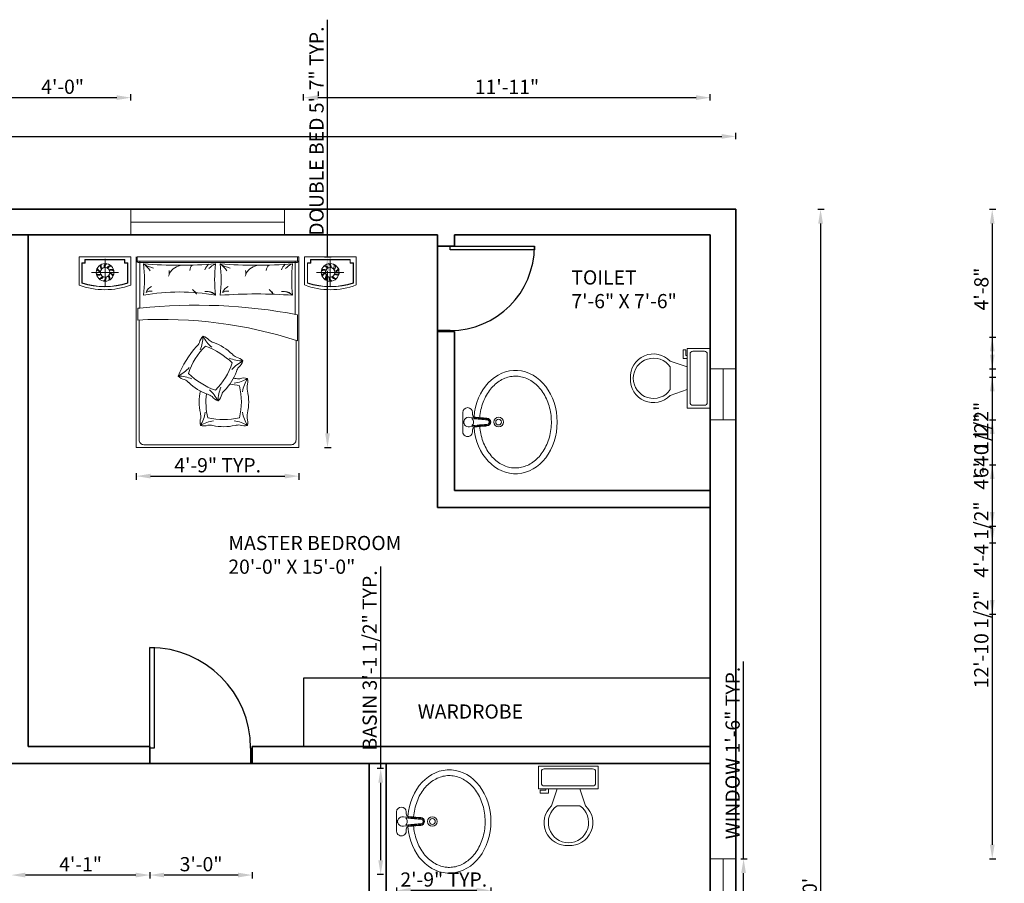
# Model space of a CAD drawing. Units: inches. Extents: x -48 to 817, y -530 to 78.
# Tile 7 of 7: x 470 to 817, y -225 to 78. Entities that reach past the tile are written whole.
import ezdxf

# ---------------------------------------------------------------- set-up
doc = ezdxf.new("R2010")
doc.units = ezdxf.units.IN
for name, color, linetype, lineweight in [('A-ANNO-DIMS', 2, 'Continuous', 18), ('A-AREA-IDEN', 7, 'Continuous', 18), ('A-DOOR', 3, 'Continuous', 25), ('A-FLOR-CASE', 8, 'Continuous', 25), ('A-FLOR-FIXT', 9, 'Continuous', 18), ('A-GLAZ', 4, 'Continuous', 18), ('A-WALL', 7, 'Continuous', 35), ('furn', 8, 'Continuous', 18), ('txt', 7, 'Continuous', 18)]:
    doc.layers.add(name, color=color, linetype=linetype, lineweight=lineweight)
doc.styles.get("Standard").update_dxf_attribs({"font": 'arial.ttf'})
doc.dimstyles.new('ISO-25', dxfattribs={"dimtxt": 5, "dimasz": 5, "dimexe": 1.25, "dimexo": 0.625, "dimtad": 1, "dimlunit": 3, "dimtxsty": 'Standard', "dimcen": 2.5, "dimadec": 0, "dimazin": 0, "dimtfac": 1, "dimtmove": 0, "dimatfit": 3, "dimfxl": 1, "dimfxlon": 1, "dimarcsym": 0})

# ---------------------------------------------------------------- blocks, each defined once
blk = doc.blocks.new('*U4')
for p, q in [((9.5, -6), (9.5, -2)), ((-10, -8.5), (-8, -8.5)), ((-10, -9.5), (-10, -8.5)), ((-7, -9.5), (-10, -9.5)), ((-8, -8.5), (-8, -8)), ((-7, -8), (-7, -9.5)), ((-4, -8), (-6, -14)), ((4, -8), (6, -14)), ((4, -14), (-4, -14))]:
    blk.add_line(p, q)
blk.add_lwpolyline([(10.5, -8), (10.5, 0), (-10.5, 0), (-10.5, -8)], close=True)
for points in [[(-9.5, -2), (-9.5, -6)], [(8.5, -1), (-8.5, -1)], [(-8.5, -7), (8.5, -7)]]:
    blk.add_lwpolyline(points)
for centre, radius, start, end in [((-8.625, -1.875), 0.8839, 81.8699, 188.1301), ((8.625, -1.875), 0.8839, 351.8699, 98.1301), ((-8.625, -6.125), 0.8839, 171.869898, 278.1301), ((8.625, -6.125), 0.8839, 261.8699, 8.1301), ((-0.4772, -19.9188), 8.0953, 133.01722, 273.38), ((0.0374, -19.8731), 7.127, 124.50543, 269.7), ((-0.0373, -19.8731), 7.127, 270.3, 55.4946), ((0.4773, -19.9188), 8.0953, 266.62, 46.9828)]:
    blk.add_arc(centre, radius, start, end)
blk = doc.blocks.new('*U2')
for p, q in [((0, 0), (0, -6)), ((40, 0), (40, -6))]:
    blk.add_line(p, q)
blk.add_lwpolyline([(0, 0), (0, 40), (1.75, 40), (1.75, 0)], close=True)
blk.add_arc((0, 0), 40, 0, 90)
blk = doc.blocks.new('A$C359865C9')
for p, q in [((0.26, 0.5858), (0.38, 0.5858)), ((0.26, 0.5258), (0.272, 0.5258)), ((0.368, 0.5258), (0.3809, 0.5258))]:
    blk.add_line(p, q)
for radius in [0.03, 0.018]:
    blk.add_circle((0.3201, 0.3632), radius)
for centre, radius, start, end in [((0.26, 0.5558), 0.03, 90.00613, 270.00613), ((0.32, 0.5495), 0.03, 348.15369, 191.84631), ((0.38, 0.5558), 0.03, 270.00613, 89.98161), ((0.272, 0.5078), 0.018, 0.00613, 90.00613), ((0.32, 0.5495), 0.03, 222.45226, 317.54774), ((0.368, 0.5078), 0.018, 90.00613, 180.00613), ((0.3201, 0.4358), 0.024, 180.00613, 0.00613), ((0.3201, 0.4358), 0.0204, 180.00613, 0.00613), ((0.3201, 0.4358), 0.0144, 180.00613, 0.00613)]:
    blk.add_arc(centre, radius, start, end)
at = {"extrusion": (0, 0, -1)}
blk.add_ellipse((0.3199, 0.5826), major_axis=(-0.00812, 0), ratio=0.392595, dxfattribs=at)
at = {"ltscale": 100, "extrusion": (0, 0, -1)}
blk.add_ellipse((0.3201, 0.258), major_axis=(0.3216, 0), ratio=0.80597, start_param=-1.471508, end_param=4.612925, dxfattribs=at)
for points, knots in [([(0.29, 0.5078), (0.2913, 0.4937), (0.2935, 0.4697), (0.2953, 0.4457), (0.2961, 0.4358)], [0, 0, 0, 0, 35.358253, 60.208758, 60.208758, 60.208758, 60.208758]), ([(0.2907, 0.5434), (0.2946, 0.498), (0.2952, 0.4908), (0.2965, 0.4761), (0.2971, 0.4686), (0.2983, 0.4536), (0.2989, 0.4461), (0.2995, 0.4378), (0.2996, 0.4369), (0.2996, 0.4361)], [2.511178, 2.511178, 2.511178, 2.511178, 20.495008, 20.495008, 39.297594, 39.297594, 58.10018, 58.10018, 60.208758, 60.208758, 60.208758, 60.208758]), ([(0.2979, 0.5293), (0.298, 0.528), (0.2981, 0.5267), (0.2988, 0.5184), (0.2993, 0.5127), (0.3005, 0.4986), (0.301, 0.4933), (0.3014, 0.4884), (0.3015, 0.4875), (0.3017, 0.4857), (0.3017, 0.485), (0.3019, 0.4827), (0.3021, 0.4812), (0.3026, 0.4756), (0.3029, 0.4716), (0.3037, 0.4621), (0.3041, 0.4568), (0.3049, 0.4464), (0.3053, 0.4415), (0.3056, 0.4365)], [4.643985, 4.643985, 4.643985, 4.643985, 5.282102, 5.282102, 8.976667, 8.976667, 16.365798, 16.365798, 18.536065, 18.536065, 20.434607, 20.434607, 24.231692, 24.231692, 34.371999, 34.371999, 47.807513, 47.807513, 60.208758, 60.208758, 60.208758, 60.208758]), ([(0.3422, 0.5293), (0.3421, 0.528), (0.342, 0.5267), (0.3412, 0.5184), (0.3408, 0.5127), (0.3395, 0.4986), (0.3391, 0.4933), (0.3387, 0.4884), (0.3386, 0.4875), (0.3384, 0.4857), (0.3383, 0.485), (0.3381, 0.4827), (0.338, 0.4812), (0.3375, 0.4756), (0.3372, 0.4716), (0.3364, 0.4621), (0.336, 0.4568), (0.3352, 0.4464), (0.3348, 0.4415), (0.3345, 0.4365)], [4.643985, 4.643985, 4.643985, 4.643985, 5.282102, 5.282102, 8.976667, 8.976667, 16.365798, 16.365798, 18.536065, 18.536065, 20.434607, 20.434607, 24.231692, 24.231692, 34.371999, 34.371999, 47.807513, 47.807513, 60.208758, 60.208758, 60.208758, 60.208758]), ([(0.3494, 0.5434), (0.3455, 0.498), (0.3449, 0.4908), (0.3436, 0.4761), (0.343, 0.4686), (0.3418, 0.4536), (0.3412, 0.4461), (0.3406, 0.4378), (0.3405, 0.4369), (0.3404, 0.4361)], [2.511178, 2.511178, 2.511178, 2.511178, 20.495008, 20.495008, 39.297594, 39.297594, 58.10018, 58.10018, 60.208758, 60.208758, 60.208758, 60.208758]), ([(0.35, 0.5078), (0.3487, 0.4937), (0.3466, 0.4697), (0.3448, 0.4457), (0.344, 0.4358)], [0, 0, 0, 0, 35.358253, 60.208758, 60.208758, 60.208758, 60.208758]), ([(0.3475, 0.4801), (0.3477, 0.4801), (0.3479, 0.4801), (0.3648, 0.4788), (0.3813, 0.4763), (0.4136, 0.4692), (0.4293, 0.4645), (0.4593, 0.4531), (0.4737, 0.4464), (0.5006, 0.4312), (0.5131, 0.4227), (0.5361, 0.4042), (0.5465, 0.3942), (0.5649, 0.3732), (0.5729, 0.3622), (0.5864, 0.3393), (0.5918, 0.3275), (0.6, 0.3036), (0.6029, 0.2914), (0.6059, 0.2669), (0.6061, 0.2545), (0.6039, 0.2301), (0.6015, 0.218), (0.5941, 0.1942), (0.5892, 0.1825), (0.5768, 0.1597), (0.5693, 0.1486), (0.552, 0.1275), (0.5422, 0.1174), (0.5203, 0.0986), (0.5083, 0.0899), (0.4825, 0.0741), (0.4686, 0.0671), (0.4396, 0.0549), (0.4243, 0.0498), (0.3929, 0.0418), (0.3767, 0.0388), (0.3439, 0.0352), (0.3273, 0.0344), (0.2942, 0.0353), (0.2776, 0.0369), (0.2452, 0.0422), (0.2293, 0.046), (0.1987, 0.0556), (0.1839, 0.0615), (0.156, 0.0751), (0.1428, 0.0828), (0.1184, 0.0997), (0.1071, 0.109), (0.0869, 0.1288), (0.078, 0.1393), (0.0625, 0.1611), (0.0559, 0.1725), (0.0454, 0.1957), (0.0415, 0.2076), (0.036, 0.2317), (0.0346, 0.2438), (0.0345, 0.2566), (0.0345, 0.2573), (0.0345, 0.258), (0.0345, 0.2664), (0.0351, 0.2749), (0.0382, 0.2956), (0.0413, 0.3078), (0.0502, 0.3317), (0.0559, 0.3434), (0.0699, 0.3661), (0.0782, 0.377), (0.0972, 0.3978), (0.1079, 0.4076), (0.1313, 0.4257), (0.1441, 0.434), (0.1714, 0.4488), (0.186, 0.4553), (0.2163, 0.4662), (0.2321, 0.4706), (0.2628, 0.4769), (0.2776, 0.479), (0.2925, 0.4801)], [1.664851, 1.664851, 1.664851, 1.664851, 1.666804, 1.666804, 1.838807, 1.838807, 2.01081, 2.01081, 2.182814, 2.182814, 2.354817, 2.354817, 2.52682, 2.52682, 2.698824, 2.698824, 2.870827, 2.870827, 3.04283, 3.04283, 3.214834, 3.214834, 3.384783, 3.384783, 3.554732, 3.554732, 3.724681, 3.724681, 3.89463, 3.89463, 4.064578, 4.064578, 4.234527, 4.234527, 4.404476, 4.404476, 4.574425, 4.574425, 4.744374, 4.744374, 4.914323, 4.914323, 5.084272, 5.084272, 5.254221, 5.254221, 5.42417, 5.42417, 5.594119, 5.594119, 5.764068, 5.764068, 5.934016, 5.934016, 6.103965, 6.103965, 6.273914, 6.273914, 6.283185, 6.283185, 6.283185, 6.401959, 6.401959, 6.573962, 6.573962, 6.745965, 6.745965, 6.917969, 6.917969, 7.089972, 7.089972, 7.261975, 7.261975, 7.433979, 7.433979, 7.605982, 7.605982, 7.759676, 7.759676, 7.759676, 7.759676])]:
    blk.add_open_spline(points, degree=3, knots=knots)
blk = doc.blocks.new('*D9')
at = {"layer": 'A-ANNO-DIMS', "color": 0, "lineweight": -2, "transparency": 16777216}
for p, q in [((2.43, 36.38), (2.43, 38.63)), ((722.43, 36.38), (722.43, 38.63)), ((7.43, 37.38), (717.43, 37.38))]:
    blk.add_line(p, q, dxfattribs=at)
at = {"layer": 'A-ANNO-DIMS', "color": 0, "transparency": 16777216}
for points in [[(7.43, 38.21), (7.43, 36.54), (2.43, 37.38)], [(717.43, 38.21), (717.43, 36.54), (722.43, 37.38)]]:
    blk.add_solid(points, dxfattribs=at)
at = {"layer": 'Defpoints', "color": 0, "transparency": 16777216}
for p in [(722.43, 37.38), (2.43, 11.72), (722.43, 11.72)]:
    blk.add_point(p, dxfattribs=at)
at = {"layer": 'A-ANNO-DIMS', "color": 0, "transparency": 16777216, "insert": (362.43, 40.55), "char_height": 5, "attachment_point": 5}
blk.add_mtext("60'", dxfattribs=at)
blk = doc.blocks.new('*D10')
at = {"layer": 'A-ANNO-DIMS', "color": 0, "lineweight": -2, "transparency": 16777216}
for p, q in [((751.22, 11.72), (753.47, 11.72)), ((752.22, 6.72), (752.22, -463.28)), ((751.22, -468.28), (753.47, -468.28))]:
    blk.add_line(p, q, dxfattribs=at)
at = {"layer": 'A-ANNO-DIMS', "color": 0, "transparency": 16777216}
for points in [[(751.39, 6.72), (753.06, 6.72), (752.22, 11.72)], [(751.39, -463.28), (753.06, -463.28), (752.22, -468.28)]]:
    blk.add_solid(points, dxfattribs=at)
at = {"layer": 'Defpoints', "color": 0, "transparency": 16777216}
for p in [(729.44, 11.72), (722.43, -468.28), (752.22, -468.28)]:
    blk.add_point(p, dxfattribs=at)
at = {"layer": 'A-ANNO-DIMS', "color": 0, "transparency": 16777216, "insert": (749.05, -228.28), "char_height": 5, "attachment_point": 5, "rotation": 90}
blk.add_mtext("40'", dxfattribs=at)
blk = doc.blocks.new('BED-DOUBLE')
for p, q in [((0.99, 65.08), (56.21, 65.08)), ((1.28, 65.57), (1.28, 49.06)), ((55.89, 65.57), (55.89, 46.91))]:
    blk.add_line(p, q)
for points in [[(0, 67.12), (0, 0), (57.2, 0), (57.2, 67.12)], [(56.67, 67.12), (56.67, 65.57), (0.33, 65.57), (0.33, 67.12), (57.2, 67.12)]]:
    blk.add_lwpolyline(points)
for points in [[(2.54, 53.57, 0.058596), (2.54, 64.62, 0.036889), (27.85, 64.62, 0.052163), (27.85, 53.57, 0.093111)], [(29.5, 53.57, 0.058596), (29.5, 64.62, 0.036648), (54.99, 64.62, 0.052163), (54.99, 53.57, 0.036967)], [(0.5, 49.06), (1.28, 49.06, -0.072944), (56.67, 46.75), (56.67, 37.58, 0.092568), (0.5, 44.85)]]:
    blk.add_lwpolyline(points, format="xyb", close=True)
for points in [[(0.99, 44.88), (0.99, 2.65, 0.414214), (2.65, 0.99), (54.56, 0.99, 0.414214), (56.21, 2.65), (56.21, 37.74)], [(22.46, 34.35, 0.091296), (23.47, 39.19, 0.091296), (26.52, 35.29, 0.091296)], [(18.37, 26.07, 0.111006), (27.81, 20.2, 0.119549), (33.77, 29.75, 0.107813), (24.35, 35.65)], [(24.3, 35.64, 0.121865), (18.37, 26.07, 0.121865)], [(32.66, 31.47, 0.091296), (37.5, 30.45, 0.091296), (33.59, 27.41, 0.091296)], [(19.57, 24.14, 0.091296), (14.72, 25.16, 0.091296), (18.63, 28.19, 0.091296)], [(28.76, 16.41, 0.159461), (30.04, 18.69, -0.076283), (31.05, 20.1, 0.115075), (35.2, 26.76, -0.076283), (36.02, 28.3, 0.159461), (37.5, 30.45)], [(34.44, 22.59, 0.091296), (39.09, 24.28, 0.091296), (37.38, 19.64, 0.091296)], [(39.09, 7.75, 0.159461), (38.98, 10.35, -0.076283), (39.09, 12.09, 0.115075), (39.09, 19.94, -0.076283), (38.98, 21.68, 0.159461), (39.09, 24.28)], [(25.17, 10.45, 0.111006), (36.29, 10.46, 0.119549), (36.29, 21.72, 0.033212), (32.87, 22.24)], [(29.76, 21.26, 0.091296), (28.76, 16.41, 0.091296), (25.71, 20.31)], [(27.21, 9.44, 0.091296), (22.56, 7.75, 0.091296), (24.27, 12.39, 0.091296)], [(37.38, 12.39, 0.091296), (39.09, 7.75, 0.091296), (34.44, 9.44)]]:
    blk.add_lwpolyline(points, format="xyb")
for centre, radius, start, end in [((0.99, 66.07), 0.992, 180, 270), ((56.21, 66.07), 0.992, 270, 0), ((8.41, 73.86), 10.95, 237.5379, 257.5233), ((-5.75, 54.29), 13.24, 36.4935, 51.2792), ((16.81, 58.07), 6.13, 96.6849, 148.3182), ((23.01, 61.56), 4.3, 141.8174, 169.8987), ((28.45, 60.95), 4.63, 130.5354, 160.3558), ((31.33, 57.05), 8.33, 114.6457, 134.1585), ((21.22, 54.29), 13.24, 36.4935, 51.2792), ((35.38, 73.86), 10.95, 237.5379, 257.5233), ((43.78, 58.07), 6.13, 96.6849, 148.3182), ((49.97, 61.56), 4.3, 141.8174, 169.8987), ((55.41, 60.95), 4.63, 130.5354, 160.3558), ((58.29, 57.05), 8.33, 114.6457, 134.1585), ((8.86, 61.48), 2.75, 335.8927, 16.1192), ((35.82, 61.48), 2.75, 335.8927, 16.1192), ((6.89, 53.32), 3.67, 114.2916, 160.9896), ((9.99, 45.89), 13.8, 36.2085, 45.0849), ((33.85, 53.32), 3.67, 114.2916, 160.9896), ((36.95, 45.89), 13.8, 36.2085, 45.0849), ((4.98, 52.55), 2.51, 76.4823, 128.5563), ((20.2, 54.04), 0.927, 353.7543, 77.2187), ((24.63, 50.41), 4.52, 44.406, 96.8342), ((25.47, 51.99), 2.86, 33.6349, 90.8456), ((31.95, 52.55), 2.51, 76.4823, 128.5563), ((47.16, 54.04), 0.927, 353.7543, 77.2187), ((51.59, 50.41), 4.52, 44.406, 96.8342), ((52.44, 51.99), 2.86, 33.6349, 90.8456), ((26.3, 36.1), 4.19, 132.4658, 168.7065), ((22.36, 35.3), 4.04, 37.2937, 74.0973), ((48.24, 11.46), 36.21, 138.3818, 157.7644), ((17.07, 39.52), 5.74, 315.5854, 333.0343), ((29.01, 42.35), 5.74, 233.2983, 250.7472), ((21.6, 20.56), 17.28, 45.1307, 71.3884), ((37.79, 36.92), 5.74, 225.7718, 243.2208), ((34.51, 27.99), 3.87, 39.4726, 79.6505), ((17.81, 28), 4.19, 222.6522, 258.8929), ((30.83, 7.48), 17.28, 77.0576, 78.7033), ((35.92, 29.93), 5.74, 257.6988, 275.1477), ((37.86, 20.61), 3.87, 71.3996, 111.5774), ((14.41, 18.76), 5.74, 45.7718, 63.2208), ((30.61, 35.12), 17.28, 225.1307, 251.3884), ((39.38, 16.01), 17.28, 166.8711, 193.1289), ((47.91, 16.13), 23.44, 173.1956, 194.0284), ((23.2, 13.33), 5.74, 53.2983, 70.7472), ((30.37, 20.93), 4.79, 218.7754, 250.3571), ((16.95, 10.85), 5.74, 355.0387, 12.4877), ((26.6, 8.88), 4.19, 159.3666, 195.6073), ((23.67, 11.79), 4.19, 254.5791, 290.8198), ((25.68, 2.15), 5.74, 77.6988, 95.1477), ((30.77, 24.6), 17.28, 257.0576, 283.3153), ((36.01, 2.19), 5.74, 85.2252, 102.6741), ((38.07, 12.43), 4.79, 250.7023, 282.284)]:
    blk.add_arc(centre, radius, start, end)
blk = doc.blocks.new('NIGHTSTAND-WITH-LAMP-L')
for p, q in [((9.19, 1.33), (9.19, 10.86)), ((4.42, 6.1), (13.95, 6.1))]:
    blk.add_line(p, q)
blk.add_lwpolyline([(0, 1.65), (0, 11.57), (18.19, 11.57), (18.19, 1.65, -0.181818)], format="xyb", close=True)
for points in [[(2.08, 10.58), (2.08, 9.49), (0.99, 9.49)], [(2.18, 10.58), (2.18, 9.39), (0.99, 9.39)], [(2.08, 10.58), (16.1, 10.58)], [(2.08, 10.48), (16.1, 10.48)], [(16, 10.58), (16, 9.39), (17.19, 9.39)], [(16.1, 10.58), (16.1, 9.49), (17.19, 9.49)]]:
    blk.add_lwpolyline(points)
for points in [[(17.19, 9.49), (17.19, 2.35, -0.167087), (0.99, 2.35), (0.99, 9.49)], [(17.09, 9.49), (17.09, 2.42, -0.165559), (1.09, 2.42), (1.09, 9.49)]]:
    blk.add_lwpolyline(points, format="xyb")
for radius in [3.11, 1.69]:
    blk.add_circle((9.19, 6.1), radius)
for centre, radius, start, end in [((8.04, 8.15), 2, 208.17, 254.4897), ((7.91, 8), 1.53, 196.3002, 256.538), ((9.46, 8.43), 2, 172.17, 218.4897), ((9.27, 8.39), 1.53, 160.3002, 220.538), ((10.78, 7.82), 2, 136.17, 182.4897), ((10.6, 7.9), 1.53, 124.3002, 184.538), ((11.49, 6.56), 2, 100.17, 146.4897), ((11.39, 6.73), 1.53, 88.3002, 148.538), ((11.32, 5.11), 2, 64.17, 110.4897), ((7.03, 6.88), 1.53, 232.3002, 292.538), ((7.05, 7.08), 2, 244.17, 290.4897), ((6.98, 5.47), 1.53, 268.3002, 328.538), ((6.88, 5.64), 2, 280.17, 326.4897), ((7.78, 4.29), 1.53, 304.3002, 4.538), ((7.59, 4.37), 2, 316.17, 2.4897), ((9.11, 3.81), 1.53, 340.3002, 40.538), ((8.91, 3.76), 2, 352.17, 38.4897), ((11.34, 5.31), 1.53, 52.3002, 112.538), ((10.47, 4.2), 1.53, 16.3002, 76.538), ((10.33, 4.05), 2, 28.17, 74.4897)]:
    blk.add_arc(centre, radius, start, end)
blk = doc.blocks.new('NIGHTSTAND-WITH-LAMP-R')
for p, q in [((9, 1.32), (9, 10.86)), ((13.77, 6.09), (4.23, 6.09))]:
    blk.add_line(p, q)
blk.add_lwpolyline([(18.19, 1.65), (18.19, 11.57), (0, 11.57), (0, 1.65, 0.181818)], format="xyb", close=True)
for points in [[(2.08, 10.58), (2.08, 9.49), (0.99, 9.49)], [(2.18, 10.58), (2.18, 9.39), (0.99, 9.39)], [(16.1, 10.58), (2.08, 10.58)], [(16.1, 10.48), (2.08, 10.48)], [(16, 10.58), (16, 9.39), (17.19, 9.39)], [(16.1, 10.58), (16.1, 9.49), (17.19, 9.49)]]:
    blk.add_lwpolyline(points)
for points in [[(0.99, 9.49), (0.99, 2.35, 0.167087), (17.19, 2.35), (17.19, 9.49)], [(1.09, 9.49), (1.09, 2.42, 0.165559), (17.09, 2.42), (17.09, 9.49)]]:
    blk.add_lwpolyline(points, format="xyb")
for radius in [3.11, 1.69]:
    blk.add_circle((9, 6.09), radius)
for centre, radius, start, end in [((6.87, 5.11), 2, 69.5103, 115.83), ((6.8, 6.72), 1.53, 31.462, 91.6998), ((6.69, 6.55), 2, 33.5103, 79.83), ((7.59, 7.9), 1.53, 355.462, 55.6998), ((7.4, 7.82), 2, 357.5103, 43.83), ((8.92, 8.38), 1.53, 319.462, 19.6998), ((8.95, 8.51), 2, 321.5103, 7.83), ((10.51, 8.08), 1.53, 283.462, 343.6998), ((10.37, 8.23), 2, 285.5103, 331.83), ((6.85, 5.31), 1.53, 67.462, 127.6998), ((7.85, 4.04), 2, 105.5103, 151.83), ((7.72, 4.19), 1.53, 103.462, 163.6998), ((9.27, 3.76), 2, 141.5103, 187.83), ((9.08, 3.8), 1.53, 139.462, 199.6998), ((10.59, 4.37), 2, 177.5103, 223.83), ((10.41, 4.29), 1.53, 175.462, 235.6998), ((11.3, 5.63), 2, 213.5103, 259.83), ((11.2, 5.46), 1.53, 211.462, 271.6998), ((11.36, 7.16), 2, 249.5103, 295.83), ((11.38, 6.96), 1.53, 247.462, 307.6998)]:
    blk.add_arc(centre, radius, start, end)
blk = doc.blocks.new('WIN-54IN')
blk.add_line((4.5, 54), (4.5, 0))
blk.add_lwpolyline([(9, 54), (0, 54), (0, 0), (9, 0)], close=True)
blk = doc.blocks.new('WIN-18IN')
blk.add_line((4.5, 18), (4.5, 0))
blk.add_lwpolyline([(0, 18), (9, 18), (9, 0), (0, 0)], close=True)
blk = doc.blocks.new('*D24')
at = {"layer": 'A-ANNO-DIMS', "color": 0, "lineweight": -2, "transparency": 16777216}
for p, q in [((725.13, -216.89), (725.13, -147.37)), ((724.13, -216.89), (726.38, -216.89)), ((725.13, -229.89), (725.13, -221.89)), ((724.13, -234.89), (726.38, -234.89))]:
    blk.add_line(p, q, dxfattribs=at)
at = {"layer": 'A-ANNO-DIMS', "color": 0, "transparency": 16777216}
for points in [[(724.29, -221.89), (725.96, -221.89), (725.13, -216.89)], [(724.29, -229.89), (725.96, -229.89), (725.13, -234.89)]]:
    blk.add_solid(points, dxfattribs=at)
at = {"layer": 'Defpoints', "color": 0, "transparency": 16777216}
for p in [(722.43, -216.89), (725.13, -216.89), (722.43, -234.89)]:
    blk.add_point(p, dxfattribs=at)
at = {"layer": 'A-ANNO-DIMS', "color": 0, "transparency": 16777216, "insert": (721.92, -179.63), "char_height": 5, "attachment_point": 5, "rotation": 90}
blk.add_mtext('WINDOW 1\'-6" TYP.', dxfattribs=at)
blk = doc.blocks.new('*D28')
at = {"layer": 'A-ANNO-DIMS', "color": 0, "lineweight": -2, "transparency": 16777216}
for p, q in [((597.45, -185.08), (597.45, -114.02)), ((598.45, -185.08), (596.2, -185.08)), ((597.45, -217.37), (597.45, -190.08)), ((598.45, -222.37), (596.2, -222.37))]:
    blk.add_line(p, q, dxfattribs=at)
at = {"layer": 'A-ANNO-DIMS', "color": 0, "transparency": 16777216}
for points in [[(596.61, -190.08), (598.28, -190.08), (597.45, -185.08)], [(596.61, -217.37), (598.28, -217.37), (597.45, -222.37)]]:
    blk.add_solid(points, dxfattribs=at)
at = {"layer": 'Defpoints', "color": 0, "transparency": 16777216}
for p in [(597.45, -185.08), (603.04, -185.08), (603.04, -222.37)]:
    blk.add_point(p, dxfattribs=at)
at = {"layer": 'A-ANNO-DIMS', "color": 0, "transparency": 16777216, "insert": (594.23, -147.05), "char_height": 5, "attachment_point": 5, "rotation": 90}
blk.add_mtext('BASIN 3\'-1 1/2" TYP.', dxfattribs=at)
blk = doc.blocks.new('*D29')
at = {"layer": 'A-ANNO-DIMS', "color": 0, "lineweight": -2, "transparency": 16777216}
for p, q in [((603.04, -226.97), (603.04, -229.22)), ((631.24, -227.97), (608.04, -227.97)), ((636.24, -226.97), (636.24, -229.22))]:
    blk.add_line(p, q, dxfattribs=at)
at = {"layer": 'A-ANNO-DIMS', "color": 0, "transparency": 16777216}
for points in [[(608.04, -227.13), (608.04, -228.8), (603.04, -227.97)], [(631.24, -227.13), (631.24, -228.8), (636.24, -227.97)]]:
    blk.add_solid(points, dxfattribs=at)
at = {"layer": 'Defpoints', "color": 0, "transparency": 16777216}
for p in [(603.04, -222.37), (636.24, -222.37), (603.04, -227.97)]:
    blk.add_point(p, dxfattribs=at)
at = {"layer": 'A-ANNO-DIMS', "color": 0, "transparency": 16777216, "insert": (619.64, -224.79), "char_height": 5, "attachment_point": 5}
blk.add_mtext('2\'-9" TYP.', dxfattribs=at)
blk = doc.blocks.new('*D32')
at = {"layer": 'A-ANNO-DIMS', "color": 0, "lineweight": -2, "transparency": 16777216}
for p, q in [((578.73, -4.99), (578.73, 78.46)), ((577.73, -4.99), (579.98, -4.99)), ((578.73, -67.11), (578.73, -9.99)), ((577.73, -72.11), (579.98, -72.11))]:
    blk.add_line(p, q, dxfattribs=at)
at = {"layer": 'A-ANNO-DIMS', "color": 0, "transparency": 16777216}
for points in [[(577.9, -9.99), (579.57, -9.99), (578.73, -4.99)], [(577.9, -67.11), (579.57, -67.11), (578.73, -72.11)]]:
    blk.add_solid(points, dxfattribs=at)
at = {"layer": 'Defpoints', "color": 0, "transparency": 16777216}
for p in [(568.67, -4.99), (578.73, -4.99), (568.67, -72.11)]:
    blk.add_point(p, dxfattribs=at)
at = {"layer": 'A-ANNO-DIMS', "color": 0, "transparency": 16777216, "insert": (575.52, 39.24), "char_height": 5, "attachment_point": 5, "rotation": 90}
blk.add_mtext('DOUBLE BED 5\'-7" TYP.', dxfattribs=at)
blk = doc.blocks.new('*D33')
at = {"layer": 'A-ANNO-DIMS', "color": 0, "lineweight": -2, "transparency": 16777216}
for p, q in [((511.46, -81.18), (511.46, -83.43)), ((516.46, -82.18), (563.67, -82.18)), ((568.67, -81.18), (568.67, -83.43))]:
    blk.add_line(p, q, dxfattribs=at)
at = {"layer": 'A-ANNO-DIMS', "color": 0, "transparency": 16777216}
for points in [[(516.46, -81.34), (516.46, -83.01), (511.46, -82.18)], [(563.67, -81.34), (563.67, -83.01), (568.67, -82.18)]]:
    blk.add_solid(points, dxfattribs=at)
at = {"layer": 'Defpoints', "color": 0, "transparency": 16777216}
for p in [(511.46, -72.11), (568.67, -72.11), (568.67, -82.18)]:
    blk.add_point(p, dxfattribs=at)
at = {"layer": 'A-ANNO-DIMS', "color": 0, "transparency": 16777216, "insert": (540.07, -79), "char_height": 5, "attachment_point": 5}
blk.add_mtext('4\'-9" TYP.', dxfattribs=at)
blk = doc.blocks.new('*D49')
at = {"layer": 'A-ANNO-DIMS', "color": 0, "lineweight": -2, "transparency": 16777216}
for p, q in [((461.47, 50.02), (461.47, 52.27)), ((509.58, 50.02), (509.58, 52.27)), ((466.47, 51.02), (504.58, 51.02))]:
    blk.add_line(p, q, dxfattribs=at)
at = {"layer": 'A-ANNO-DIMS', "color": 0, "transparency": 16777216}
for points in [[(466.47, 51.86), (466.47, 50.19), (461.47, 51.02)], [(504.58, 51.86), (504.58, 50.19), (509.58, 51.02)]]:
    blk.add_solid(points, dxfattribs=at)
at = {"layer": 'Defpoints', "color": 0, "transparency": 16777216}
for p in [(509.58, 51.02), (461.47, 11.72), (509.58, 11.72)]:
    blk.add_point(p, dxfattribs=at)
at = {"layer": 'A-ANNO-DIMS', "color": 0, "transparency": 16777216, "insert": (485.53, 54.2), "char_height": 5, "attachment_point": 5}
blk.add_mtext('4\'-0"', dxfattribs=at)
blk = doc.blocks.new('*D53')
at = {"layer": 'A-ANNO-DIMS', "color": 0, "lineweight": -2, "transparency": 16777216}
for p, q in [((811.62, 11.72), (813.87, 11.72)), ((812.62, 6.72), (812.62, -39.41)), ((811.62, -44.41), (813.87, -44.41))]:
    blk.add_line(p, q, dxfattribs=at)
at = {"layer": 'A-ANNO-DIMS', "color": 0, "transparency": 16777216}
for points in [[(811.79, 6.72), (813.45, 6.72), (812.62, 11.72)], [(811.79, -39.41), (813.45, -39.41), (812.62, -44.41)]]:
    blk.add_solid(points, dxfattribs=at)
at = {"layer": 'Defpoints', "color": 0, "transparency": 16777216}
for p in [(722.43, 11.72), (722.43, -44.41), (812.62, -44.41)]:
    blk.add_point(p, dxfattribs=at)
at = {"layer": 'A-ANNO-DIMS', "color": 0, "transparency": 16777216, "insert": (809.44, -16.34), "char_height": 5, "attachment_point": 5, "rotation": 90}
blk.add_mtext('4\'-8"', dxfattribs=at)
blk = doc.blocks.new('*D54')
at = {"layer": 'A-ANNO-DIMS', "color": 0, "lineweight": -2, "transparency": 16777216}
for p, q in [((811.62, -62.41), (813.87, -62.41)), ((812.62, -67.41), (812.62, -211.89)), ((811.62, -216.89), (813.87, -216.89))]:
    blk.add_line(p, q, dxfattribs=at)
at = {"layer": 'A-ANNO-DIMS', "color": 0, "transparency": 16777216}
for points in [[(811.79, -67.41), (813.45, -67.41), (812.62, -62.41)], [(811.79, -211.89), (813.45, -211.89), (812.62, -216.89)]]:
    blk.add_solid(points, dxfattribs=at)
at = {"layer": 'Defpoints', "color": 0, "transparency": 16777216}
for p in [(722.43, -62.41), (722.43, -216.89), (812.62, -216.89)]:
    blk.add_point(p, dxfattribs=at)
at = {"layer": 'A-ANNO-DIMS', "color": 0, "transparency": 16777216, "insert": (809.41, -139.65), "char_height": 5, "attachment_point": 5, "rotation": 90}
blk.add_mtext('12\'-10 1/2"', dxfattribs=at)
blk = doc.blocks.new('*D58')
at = {"layer": 'A-ANNO-DIMS', "color": 0, "lineweight": -2, "transparency": 16777216}
for p, q in [((811.62, -33.28), (813.87, -33.28)), ((812.62, -38.28), (812.62, -100.61)), ((811.62, -105.61), (813.87, -105.61))]:
    blk.add_line(p, q, dxfattribs=at)
at = {"layer": 'A-ANNO-DIMS', "color": 0, "transparency": 16777216}
for points in [[(811.79, -38.28), (813.45, -38.28), (812.62, -33.28)], [(811.79, -100.61), (813.45, -100.61), (812.62, -105.61)]]:
    blk.add_solid(points, dxfattribs=at)
at = {"layer": 'Defpoints', "color": 0, "transparency": 16777216}
for p in [(161.43, -33.28), (161.43, -105.61), (812.62, -105.61)]:
    blk.add_point(p, dxfattribs=at)
at = {"layer": 'A-ANNO-DIMS', "color": 0, "transparency": 16777216, "insert": (809.41, -69.44), "char_height": 5, "attachment_point": 5, "rotation": 90}
blk.add_mtext('6\'-0 1/2"', dxfattribs=at)
blk = doc.blocks.new('*D60')
at = {"layer": 'A-ANNO-DIMS', "color": 0, "lineweight": -2, "transparency": 16777216}
for p, q in [((467.43, -221.58), (467.43, -223.83)), ((516.25, -221.58), (516.25, -223.83)), ((511.25, -222.58), (472.43, -222.58))]:
    blk.add_line(p, q, dxfattribs=at)
at = {"layer": 'A-ANNO-DIMS', "color": 0, "transparency": 16777216}
for points in [[(472.43, -221.74), (472.43, -223.41), (467.43, -222.58)], [(511.25, -221.74), (511.25, -223.41), (516.25, -222.58)]]:
    blk.add_solid(points, dxfattribs=at)
at = {"layer": 'Defpoints', "color": 0, "transparency": 16777216}
for p in [(467.43, -183.28), (516.25, -183.28), (467.43, -222.58)]:
    blk.add_point(p, dxfattribs=at)
at = {"layer": 'A-ANNO-DIMS', "color": 0, "transparency": 16777216, "insert": (491.84, -219.44), "char_height": 5, "attachment_point": 5}
blk.add_mtext('4\'-1"', dxfattribs=at)
blk = doc.blocks.new('*D61')
at = {"layer": 'A-ANNO-DIMS', "color": 0, "lineweight": -2, "transparency": 16777216}
for p, q in [((516.25, -221.58), (516.25, -223.83)), ((552.25, -221.58), (552.25, -223.83)), ((547.25, -222.58), (521.25, -222.58))]:
    blk.add_line(p, q, dxfattribs=at)
at = {"layer": 'A-ANNO-DIMS', "color": 0, "transparency": 16777216}
for points in [[(521.25, -221.74), (521.25, -223.41), (516.25, -222.58)], [(547.25, -221.74), (547.25, -223.41), (552.25, -222.58)]]:
    blk.add_solid(points, dxfattribs=at)
at = {"layer": 'Defpoints', "color": 0, "transparency": 16777216}
for p in [(516.25, -183.28), (552.25, -183.28), (516.25, -222.58)]:
    blk.add_point(p, dxfattribs=at)
at = {"layer": 'A-ANNO-DIMS', "color": 0, "transparency": 16777216, "insert": (534.25, -219.4), "char_height": 5, "attachment_point": 5}
blk.add_mtext('3\'-0"', dxfattribs=at)
blk = doc.blocks.new('*D67')
at = {"layer": 'A-ANNO-DIMS', "color": 0, "lineweight": -2, "transparency": 16777216}
for p, q in [((570.33, 50.02), (570.33, 52.27)), ((713.43, 50.02), (713.43, 52.27)), ((575.33, 51.02), (708.43, 51.02))]:
    blk.add_line(p, q, dxfattribs=at)
at = {"layer": 'A-ANNO-DIMS', "color": 0, "transparency": 16777216}
for points in [[(575.33, 51.86), (575.33, 50.19), (570.33, 51.02)], [(708.43, 51.86), (708.43, 50.19), (713.43, 51.02)]]:
    blk.add_solid(points, dxfattribs=at)
at = {"layer": 'Defpoints', "color": 0, "transparency": 16777216}
for p in [(713.43, 51.02), (570.33, -153.28), (713.43, -153.28)]:
    blk.add_point(p, dxfattribs=at)
at = {"layer": 'A-ANNO-DIMS', "color": 0, "transparency": 16777216, "insert": (641.88, 54.16), "char_height": 5, "attachment_point": 5}
blk.add_mtext('11\'-11"', dxfattribs=at)
blk = doc.blocks.new('*D68')
at = {"layer": 'A-ANNO-DIMS', "color": 0, "lineweight": -2, "transparency": 16777216}
for p, q in [((-35.87, -153.28), (-38.12, -153.28)), ((-36.87, -158.28), (-36.87, -172.28)), ((-35.87, -177.28), (-38.12, -177.28))]:
    blk.add_line(p, q, dxfattribs=at)
at = {"layer": 'A-ANNO-DIMS', "color": 0, "transparency": 16777216}
for points in [[(-37.71, -158.28), (-36.04, -158.28), (-36.87, -153.28)], [(-37.71, -172.28), (-36.04, -172.28), (-36.87, -177.28)]]:
    blk.add_solid(points, dxfattribs=at)
at = {"layer": 'Defpoints', "color": 0, "transparency": 16777216}
for p in [(570.33, -153.28), (-36.87, -177.28), (570.33, -177.28)]:
    blk.add_point(p, dxfattribs=at)
at = {"layer": 'A-ANNO-DIMS', "color": 0, "transparency": 16777216, "insert": (-40.05, -165.28), "char_height": 5, "attachment_point": 5, "rotation": 90}
blk.add_mtext('2\'-0"', dxfattribs=at)
blk = doc.blocks.new('*D74')
at = {"layer": 'A-ANNO-DIMS', "color": 0, "lineweight": -2, "transparency": 16777216}
for p, q in [((811.62, -47.3), (813.87, -47.3)), ((812.62, -52.3), (812.62, -94.77)), ((811.62, -99.77), (813.87, -99.77))]:
    blk.add_line(p, q, dxfattribs=at)
at = {"layer": 'A-ANNO-DIMS', "color": 0, "transparency": 16777216}
for points in [[(811.79, -52.3), (813.45, -52.3), (812.62, -47.3)], [(811.79, -94.77), (813.45, -94.77), (812.62, -99.77)]]:
    blk.add_solid(points, dxfattribs=at)
at = {"layer": 'Defpoints', "color": 0, "transparency": 16777216}
for p in [(44.85, -47.3), (44.85, -99.77), (812.62, -99.77)]:
    blk.add_point(p, dxfattribs=at)
at = {"layer": 'A-ANNO-DIMS', "color": 0, "transparency": 16777216, "insert": (809.41, -73.53), "char_height": 5, "attachment_point": 5, "rotation": 90}
blk.add_mtext('4\'-4 1/2"', dxfattribs=at)
blk = doc.blocks.new('*D76')
at = {"layer": 'A-ANNO-DIMS', "color": 0, "lineweight": -2, "transparency": 16777216}
for p, q in [((811.62, -78.22), (813.87, -78.22)), ((812.62, -83.22), (812.62, -125.76)), ((811.62, -130.76), (813.87, -130.76))]:
    blk.add_line(p, q, dxfattribs=at)
at = {"layer": 'A-ANNO-DIMS', "color": 0, "transparency": 16777216}
for points in [[(811.79, -83.22), (813.45, -83.22), (812.62, -78.22)], [(811.79, -125.76), (813.45, -125.76), (812.62, -130.76)]]:
    blk.add_solid(points, dxfattribs=at)
at = {"layer": 'Defpoints', "color": 0, "transparency": 16777216}
for p in [(332.6, -78.22), (332.6, -130.76), (812.62, -130.76)]:
    blk.add_point(p, dxfattribs=at)
at = {"layer": 'A-ANNO-DIMS', "color": 0, "transparency": 16777216, "insert": (809.41, -104.49), "char_height": 5, "attachment_point": 5, "rotation": 90}
blk.add_mtext('4\'-4 1/2"', dxfattribs=at)
blk = doc.blocks.new('*D81')
at = {"layer": 'A-ANNO-DIMS', "color": 0, "lineweight": -2, "transparency": 16777216}
for p, q in [((685.32, -506.59), (685.32, -508.84)), ((690.32, -507.59), (708.32, -507.59)), ((713.32, -506.59), (713.32, -508.84))]:
    blk.add_line(p, q, dxfattribs=at)
at = {"layer": 'A-ANNO-DIMS', "color": 0, "transparency": 16777216}
for points in [[(690.32, -506.76), (690.32, -508.42), (685.32, -507.59)], [(708.32, -506.76), (708.32, -508.42), (713.32, -507.59)]]:
    blk.add_solid(points, dxfattribs=at)
at = {"layer": 'Defpoints', "color": 0, "transparency": 16777216}
for p in [(685.32, -47.75), (713.32, -58.25), (713.32, -507.59)]:
    blk.add_point(p, dxfattribs=at)
at = {"layer": 'A-ANNO-DIMS', "color": 0, "transparency": 16777216, "insert": (699.32, -504.45), "char_height": 5, "attachment_point": 5}
blk.add_mtext('2\'-4"', dxfattribs=at)
blk = doc.blocks.new('*D82')
at = {"layer": 'A-ANNO-DIMS', "color": 0, "lineweight": -2, "transparency": 16777216}
for p, q in [((-35.87, -37.25), (-38.12, -37.25)), ((-36.87, -42.25), (-36.87, -53.25)), ((-35.87, -58.25), (-38.12, -58.25))]:
    blk.add_line(p, q, dxfattribs=at)
at = {"layer": 'A-ANNO-DIMS', "color": 0, "transparency": 16777216}
for points in [[(-37.71, -42.25), (-36.04, -42.25), (-36.87, -37.25)], [(-37.71, -53.25), (-36.04, -53.25), (-36.87, -58.25)]]:
    blk.add_solid(points, dxfattribs=at)
at = {"layer": 'Defpoints', "color": 0, "transparency": 16777216}
for p in [(705.32, -37.25), (-36.87, -58.25), (705.32, -58.25)]:
    blk.add_point(p, dxfattribs=at)
at = {"layer": 'A-ANNO-DIMS', "color": 0, "transparency": 16777216, "insert": (-40.05, -47.75), "char_height": 5, "attachment_point": 5, "rotation": 90}
blk.add_mtext('1\'-9"', dxfattribs=at)
blk = doc.blocks.new('*D83')
at = {"layer": 'A-ANNO-DIMS', "color": 0, "lineweight": -2, "transparency": 16777216}
for p, q in [((-35.87, -1.28), (-38.12, -1.28)), ((-36.87, -26.28), (-36.87, -6.28)), ((-35.87, -31.28), (-38.12, -31.28))]:
    blk.add_line(p, q, dxfattribs=at)
at = {"layer": 'A-ANNO-DIMS', "color": 0, "transparency": 16777216}
for points in [[(-37.71, -6.28), (-36.04, -6.28), (-36.87, -1.28)], [(-37.71, -26.28), (-36.04, -26.28), (-36.87, -31.28)]]:
    blk.add_solid(points, dxfattribs=at)
at = {"layer": 'Defpoints', "color": 0, "transparency": 16777216}
for p in [(-36.87, -1.28), (617.43, -1.28), (617.43, -31.28)]:
    blk.add_point(p, dxfattribs=at)
at = {"layer": 'A-ANNO-DIMS', "color": 0, "transparency": 16777216, "insert": (-40.05, -16.28), "char_height": 5, "attachment_point": 5, "rotation": 90}
blk.add_mtext('2\'-6"', dxfattribs=at)

msp = doc.modelspace()

# ---------------------------------------------------------------- linework, layer by layer
at = {"layer": 'A-FLOR-CASE'}
for p, q in [((713.427, -153.275), (570.327, -153.275)), ((570.327, -153.275), (570.327, -177.275))]:
    msp.add_line(p, q, dxfattribs=at)
at = {"layer": 'A-WALL'}
for p, q in [((2.427, 11.725), (722.427, 11.725)), ((722.427, 11.725), (722.427, -468.275)), ((459.913, 2.725), (473.427, 2.725)), ((473.427, 2.725), (473.427, -177.275)), ((473.427, 2.725), (617.427, 2.725)), ((617.427, 2.725), (617.427, -87.275)), ((623.427, 2.725), (623.427, -1.275)), ((623.427, 2.725), (713.427, 2.725)), ((713.427, 2.725), (713.427, -459.275)), ((623.427, -1.275), (617.427, -1.275)), ((623.427, -31.275), (617.427, -31.275)), ((623.427, -31.275), (623.427, -87.275)), ((617.427, -87.275), (617.427, -93.275)), ((623.427, -87.275), (713.427, -87.275)), ((617.427, -93.275), (713.427, -93.275)), ((473.427, -177.275), (516.248, -177.275)), ((516.248, -183.275), (516.248, -177.275)), ((552.248, -183.275), (552.248, -177.275)), ((552.248, -177.275), (713.427, -177.275)), ((473.427, -183.275), (467.427, -183.275)), ((473.427, -183.275), (713.427, -183.275)), ((593.427, -183.275), (593.427, -273.275)), ((599.427, -183.275), (599.427, -239.275))]:
    msp.add_line(p, q, dxfattribs=at)

# ---------------------------------------------------------------- block references
at = {"layer": 'A-DOOR', "xscale": 0.7416502636543669, "yscale": 0.7416502636543669, "zscale": 0.7416502636543669, "rotation": 270}
msp.add_blockref('*U2', (621.877, -1.275), dxfattribs=at)
at = {"layer": 'A-DOOR', "xscale": 0.886149626865359, "yscale": 0.886149626865359, "zscale": 0.886149626865359}
msp.add_blockref('*U2', (516.248, -177.958), dxfattribs=at)
at = {"layer": 'A-FLOR-FIXT', "rotation": 270}
msp.add_blockref('*U4', (713.322, -47.749), dxfattribs=at)
at = {"layer": 'A-FLOR-FIXT', "xscale": 56.55191473266222, "yscale": 56.55191473266222, "zscale": 56.55191473266222, "rotation": 90}
for p in [(659.469, -81.265), (636.169, -221.826)]:
    msp.add_blockref('A$C359865C9', p, dxfattribs=at)
at = {"layer": 'A-FLOR-FIXT'}
msp.add_blockref('*U4', (663.521, -184.223), dxfattribs=at)
at = {"layer": 'A-GLAZ', "rotation": 270}
msp.add_blockref('WIN-54IN', (509.583, 11.725), dxfattribs=at)
at = {"layer": 'A-GLAZ'}
for p in [(713.427, -62.413), (713.427, -234.886)]:
    msp.add_blockref('WIN-18IN', p, dxfattribs=at)
at = {"layer": 'furn'}
for name, p in [('NIGHTSTAND-WITH-LAMP-L', (491.295, -16.565)), ('BED-DOUBLE', (511.464, -72.109)), ('NIGHTSTAND-WITH-LAMP-R', (570.65, -16.562))]:
    msp.add_blockref(name, p, dxfattribs=at)

# ---------------------------------------------------------------- texts
at = {"layer": 'A-AREA-IDEN', "char_height": 5, "attachment_point": 1}
for s, width, insert in [('TOILET\\P7\'-6" X 7\'-6"', 39.91595, (664.532, -9.753)), ('MASTER BEDROOM\\P20\'-0" X 15\'-0"', 73.74706, (543.841, -103.217))]:
    msp.add_mtext_dynamic_manual_height_columns(s, width=width, gutter_width=12.5, heights=[0], dxfattribs=dict(at, insert=insert))
at = {"layer": 'txt', "insert": (610.468, -162.519), "char_height": 5, "attachment_point": 1}
msp.add_mtext_dynamic_manual_height_columns('WARDROBE', width=73.16203, gutter_width=12.5, heights=[0], dxfattribs=at)

# ---------------------------------------------------------------- dimensions: what is measured, and where the dimension line sits
at = {"layer": 'A-ANNO-DIMS'}
for base, p1, p2, angle, text, picture, middle in [((578.734, -4.988), (568.666, -72.109), (568.666, -4.988), 90, 'DOUBLE BED <> TYP.', '*D32', (575.522, 39.235)), ((597.446, -185.08), (603.04, -222.372), (603.04, -185.08), 90, 'BASIN <> TYP.', '*D28', (594.234, -147.051)), ((725.127, -216.886), (722.427, -234.886), (722.427, -216.886), 90, 'WINDOW <> TYP.', '*D24', (721.915, -179.626)), ((603.04, -227.966), (636.24, -222.372), (603.04, -222.372), 180, '<> TYP.', '*D29', (619.64, -224.788))]:
    dim = msp.add_linear_dim(base=base, p1=p1, p2=p2, angle=angle, text=text, dimstyle='ISO-25', override={"dimdec": 1, "dimlfac": 1, "dimrnd": 0, "dimzin": 1, "dimdsep": 46, "dimlunit": 4, "dimfrac": 2}, dxfattribs=at)
    dim.commit()
    dim.dimension.update_dxf_attribs({"geometry": picture, "text_midpoint": middle})
for base, p1, p2, override, picture, middle in [((509.583, 51.025), (461.475, 11.725), (509.583, 11.725), {"dimdec": 1, "dimlfac": 1, "dimrnd": 0, "dimzin": 1, "dimdsep": 46, "dimlunit": 4, "dimfrac": 2}, '*D49', (485.529, 54.202)), ((713.427, 51.025), (570.327, -153.275), (713.427, -153.275), {"dimdec": 1, "dimlfac": 1, "dimrnd": 0, "dimzin": 1, "dimdsep": 46, "dimlunit": 4, "dimfrac": 2}, '*D67', (641.877, 54.16)), ((722.427, 37.377), (2.427, 11.725), (722.427, 11.725), {"dimclrd": 0, "dimclre": 0, "dimclrt": 0}, '*D9', (362.427, 40.554)), ((713.322, -507.589), (685.322, -47.749), (713.322, -58.249), {"dimdec": 1, "dimlfac": 1, "dimrnd": 0, "dimzin": 1, "dimdsep": 46, "dimlunit": 4, "dimfrac": 2}, '*D81', (699.322, -504.454))]:
    dim = msp.add_linear_dim(base=base, p1=p1, p2=p2, dimstyle='ISO-25', override=override, dxfattribs=at)
    dim.commit()
    dim.dimension.update_dxf_attribs({"geometry": picture, "text_midpoint": middle})
for base, p1, p2, angle, override, picture, middle in [((752.224, -468.275), (729.44, 11.725), (722.427, -468.275), 90, {"dimclrd": 0, "dimclre": 0, "dimclrt": 0}, '*D10', (749.046, -228.275)), ((812.622, -44.413), (722.427, 11.725), (722.427, -44.413), 90, {"dimdec": 1, "dimlfac": 1, "dimrnd": 0, "dimzin": 1, "dimdsep": 46, "dimlunit": 4, "dimfrac": 2}, '*D53', (809.444, -16.344)), ((-36.873, -1.275), (617.427, -31.275), (617.427, -1.275), 90, {"dimdec": 1, "dimlfac": 1, "dimrnd": 0, "dimzin": 1, "dimdsep": 46, "dimlunit": 4, "dimfrac": 2}, '*D83', (-40.051, -16.275)), ((812.622, -105.612), (161.427, -33.275), (161.427, -105.612), 90, {"dimdec": 1, "dimlfac": 1, "dimrnd": 0, "dimzin": 1, "dimdsep": 46, "dimlunit": 4, "dimfrac": 2}, '*D58', (809.411, -69.444)), ((-36.873, -58.249), (705.322, -37.249), (705.322, -58.249), 90, {"dimdec": 1, "dimlfac": 1, "dimrnd": 0, "dimzin": 1, "dimdsep": 46, "dimlunit": 4, "dimfrac": 2}, '*D82', (-40.051, -47.749)), ((812.622, -99.767), (44.85, -47.302), (44.85, -99.767), 90, {"dimdec": 1, "dimlfac": 1, "dimrnd": 0, "dimzin": 1, "dimdsep": 46, "dimlunit": 4, "dimfrac": 2}, '*D74', (809.411, -73.535)), ((812.622, -216.886), (722.427, -62.413), (722.427, -216.886), 90, {"dimdec": 1, "dimlfac": 1, "dimrnd": 0, "dimzin": 1, "dimdsep": 46, "dimlunit": 4, "dimfrac": 2}, '*D54', (809.411, -139.65)), ((812.622, -130.757), (332.597, -78.216), (332.597, -130.757), 90, {"dimdec": 1, "dimlfac": 1, "dimrnd": 0, "dimzin": 1, "dimdsep": 46, "dimlunit": 4, "dimfrac": 2}, '*D76', (809.411, -104.487)), ((-36.873, -177.275), (570.327, -153.275), (570.327, -177.275), 90, {"dimdec": 1, "dimlfac": 1, "dimrnd": 0, "dimzin": 1, "dimdsep": 46, "dimlunit": 4, "dimfrac": 2}, '*D68', (-40.051, -165.275)), ((467.427, -222.575), (516.248, -183.275), (467.427, -183.275), 180, {"dimdec": 1, "dimlfac": 1, "dimrnd": 0, "dimzin": 1, "dimdsep": 46, "dimlunit": 4, "dimfrac": 2}, '*D60', (491.838, -219.44)), ((516.248, -222.575), (552.248, -183.275), (516.248, -183.275), 180, {"dimdec": 1, "dimlfac": 1, "dimrnd": 0, "dimzin": 1, "dimdsep": 46, "dimlunit": 4, "dimfrac": 2}, '*D61', (534.248, -219.396))]:
    dim = msp.add_linear_dim(base=base, p1=p1, p2=p2, angle=angle, dimstyle='ISO-25', override=override, dxfattribs=at)
    dim.commit()
    dim.dimension.update_dxf_attribs({"geometry": picture, "text_midpoint": middle})
dim = msp.add_linear_dim(base=(568.666, -82.177), p1=(511.464, -72.109), p2=(568.666, -72.109), text='<> TYP.', dimstyle='ISO-25', override={"dimdec": 1, "dimlfac": 1, "dimrnd": 0, "dimzin": 1, "dimdsep": 46, "dimlunit": 4, "dimfrac": 2}, dxfattribs=at)
dim.commit()
dim.dimension.update_dxf_attribs({"geometry": '*D33', "text_midpoint": (540.065, -78.999)})

doc.saveas('drawing.dxf')
